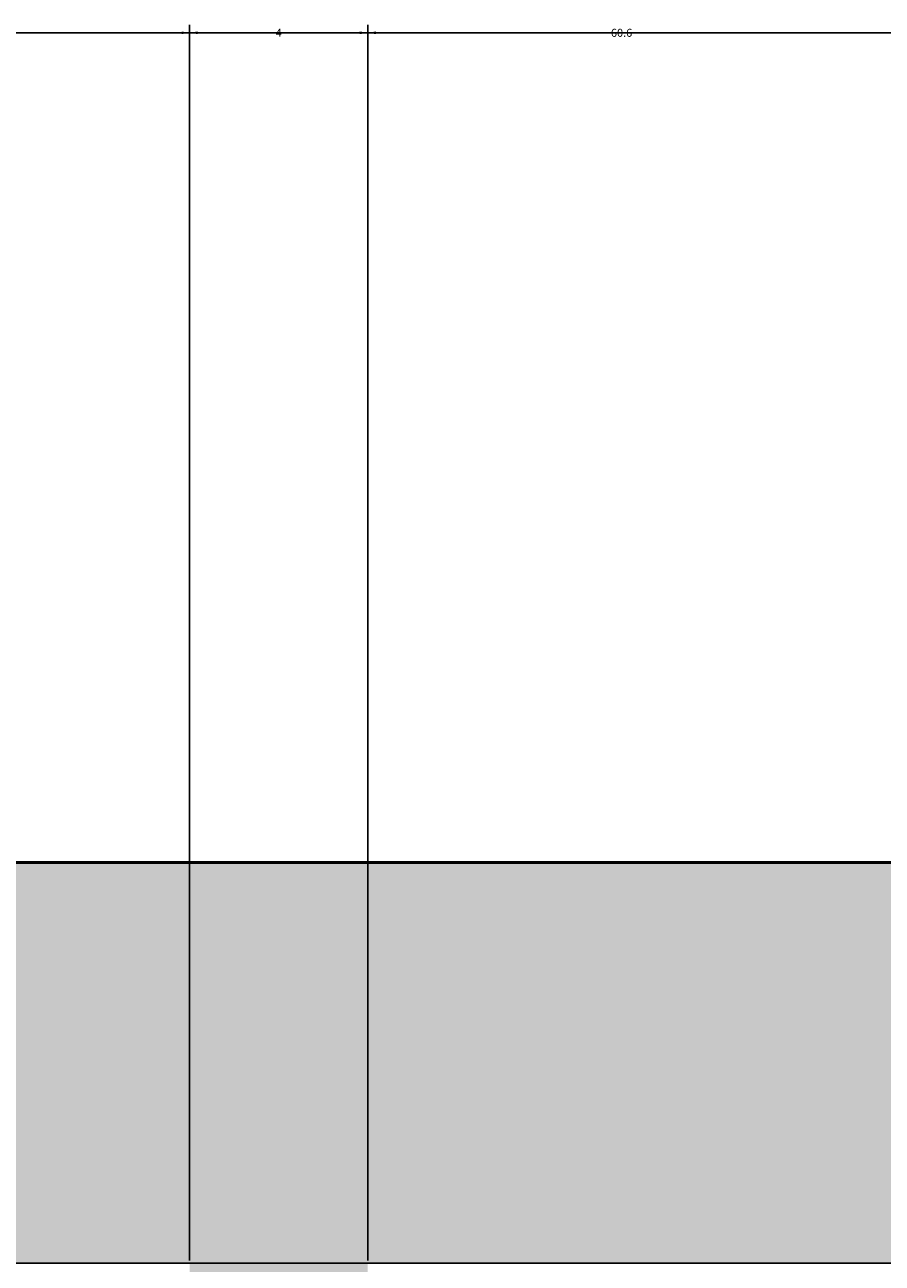
# Model space of a CAD drawing. Units: inches. Extents: x 2231 to 2461, y 2045 to 2455.
# Tile 88 of 95: x 2365 to 2384, y 2427 to 2455. Entities that reach past the tile are written whole.
import ezdxf

# ---------------------------------------------------------------- set-up
doc = ezdxf.new("R2010")
doc.units = ezdxf.units.IN
doc.layers.add('A-ANNO-DIMS', color=2, linetype='Continuous', lineweight=18)
doc.layers.add('A-WALL', color=7, linetype='Continuous', lineweight=50)
doc.layers.add('A-WALL-PATT', color=18, linetype='Continuous', lineweight=13, true_color=0x000000)
doc.styles.get("Standard").update_dxf_attribs({"font": 'arial.ttf'})
doc.dimstyles.get("Standard").update_dxf_attribs({"dimtxt": 0.18, "dimasz": 0.18, "dimexe": 0.18, "dimexo": 0.0625, "dimgap": 0.09, "dimtad": 0, "dimtih": 1, "dimtoh": 1, "dimdec": 4, "dimzin": 0, "dimdsep": 46, "dimtxsty": 'Standard', "dimcen": 0.09, "dimadec": 0, "dimazin": 0, "dimtfac": 1, "dimtdec": 4, "dimtofl": 0, "dimtmove": 0, "dimatfit": 3, "dimfxl": 1, "dimtolj": 1, "dimtzin": 0, "dimarcsym": 0})

# ---------------------------------------------------------------- blocks, each defined once
blk = doc.blocks.new('*D35')
at = {"layer": 'A-ANNO-DIMS', "color": 0, "lineweight": -2, "transparency": 16777216}
for p, q in [((2258.794, 2426.895), (2258.794, 2454.645)), ((2258.974, 2454.465), (2313.513, 2454.465)), ((2368.614, 2454.465), (2314.074, 2454.465)), ((2368.794, 2426.895), (2368.794, 2454.645))]:
    blk.add_line(p, q, dxfattribs=at)
at = {"layer": 'A-ANNO-DIMS', "color": 0, "transparency": 16777216}
for points in [[(2258.974, 2454.495), (2258.974, 2454.435), (2258.794, 2454.465)], [(2368.614, 2454.495), (2368.614, 2454.435), (2368.794, 2454.465)]]:
    blk.add_solid(points, dxfattribs=at)
at = {"layer": 'Defpoints', "color": 0, "transparency": 16777216}
for p in [(2368.794, 2454.465), (2258.794, 2426.833), (2368.794, 2426.833)]:
    blk.add_point(p, dxfattribs=at)
at = {"layer": 'A-ANNO-DIMS', "color": 0, "transparency": 16777216, "insert": (2313.794, 2454.465), "char_height": 0.18, "attachment_point": 5}
blk.add_mtext('\\A1;110', dxfattribs=at)
blk = doc.blocks.new('*D36')
at = {"layer": 'A-ANNO-DIMS', "color": 0, "lineweight": -2, "transparency": 16777216}
for p, q in [((2372.794, 2426.895), (2372.794, 2454.645)), ((2372.974, 2454.465), (2402.574, 2454.465)), ((2432.614, 2454.465), (2403.013, 2454.465)), ((2432.794, 2426.895), (2432.794, 2454.645))]:
    blk.add_line(p, q, dxfattribs=at)
at = {"layer": 'A-ANNO-DIMS', "color": 0, "transparency": 16777216}
for points in [[(2372.974, 2454.495), (2372.974, 2454.435), (2372.794, 2454.465)], [(2432.614, 2454.495), (2432.614, 2454.435), (2432.794, 2454.465)]]:
    blk.add_solid(points, dxfattribs=at)
at = {"layer": 'Defpoints', "color": 0, "transparency": 16777216}
for p in [(2432.794, 2454.465), (2372.794, 2426.833), (2432.794, 2426.833)]:
    blk.add_point(p, dxfattribs=at)
at = {"layer": 'A-ANNO-DIMS', "color": 0, "transparency": 16777216, "insert": (2402.794, 2454.465), "char_height": 0.18, "attachment_point": 5}
blk.add_mtext('\\A1;60', dxfattribs=at)
blk = doc.blocks.new('*D66')
at = {"layer": 'A-ANNO-DIMS', "color": 0, "lineweight": -2, "transparency": 16777216}
for p, q in [((2348.189, 2096.895), (2348.189, 2454.645)), ((2348.369, 2454.465), (2378.167, 2454.465)), ((2408.614, 2454.465), (2378.815, 2454.465)), ((2408.794, 2096.895), (2408.794, 2454.645))]:
    blk.add_line(p, q, dxfattribs=at)
at = {"layer": 'A-ANNO-DIMS', "color": 0, "transparency": 16777216}
for points in [[(2348.369, 2454.495), (2348.369, 2454.435), (2348.189, 2454.465)], [(2408.614, 2454.495), (2408.614, 2454.435), (2408.794, 2454.465)]]:
    blk.add_solid(points, dxfattribs=at)
at = {"layer": 'Defpoints', "color": 0, "transparency": 16777216}
for p in [(2408.794, 2454.465), (2348.189, 2096.833), (2408.794, 2096.833)]:
    blk.add_point(p, dxfattribs=at)
at = {"layer": 'A-ANNO-DIMS', "color": 0, "transparency": 16777216, "insert": (2378.491, 2454.465), "char_height": 0.18, "attachment_point": 5}
blk.add_mtext('\\A1;60.6', dxfattribs=at)
blk = doc.blocks.new('*D68')
at = {"layer": 'A-ANNO-DIMS', "color": 0, "lineweight": -2, "transparency": 16777216}
for p, q in [((2285.882, 2426.833), (2460.606, 2426.833)), ((2460.426, 2426.653), (2460.426, 2420.225)), ((2460.426, 2413.433), (2460.426, 2419.861)), ((2278.251, 2413.253), (2460.606, 2413.253))]:
    blk.add_line(p, q, dxfattribs=at)
at = {"layer": 'A-ANNO-DIMS', "color": 0, "transparency": 16777216}
for points in [[(2460.396, 2426.653), (2460.456, 2426.653), (2460.426, 2426.833)], [(2460.396, 2413.433), (2460.456, 2413.433), (2460.426, 2413.253)]]:
    blk.add_solid(points, dxfattribs=at)
at = {"layer": 'Defpoints', "color": 0, "transparency": 16777216}
for p in [(2285.82, 2426.833), (2460.426, 2426.833), (2278.188, 2413.253)]:
    blk.add_point(p, dxfattribs=at)
at = {"layer": 'A-ANNO-DIMS', "color": 0, "transparency": 16777216, "insert": (2460.426, 2420.043), "char_height": 0.18, "attachment_point": 5}
blk.add_mtext('\\A1;13.58', dxfattribs=at)
blk = doc.blocks.new('*D70')
at = {"layer": 'A-ANNO-DIMS', "color": 0, "lineweight": -2, "transparency": 16777216}
for p, q in [((2368.794, 2426.895), (2368.794, 2454.645)), ((2368.974, 2454.465), (2370.641, 2454.465)), ((2372.614, 2454.465), (2370.946, 2454.465)), ((2372.794, 2426.895), (2372.794, 2454.645))]:
    blk.add_line(p, q, dxfattribs=at)
at = {"layer": 'A-ANNO-DIMS', "color": 0, "transparency": 16777216}
for points in [[(2368.974, 2454.495), (2368.974, 2454.435), (2368.794, 2454.465)], [(2372.614, 2454.495), (2372.614, 2454.435), (2372.794, 2454.465)]]:
    blk.add_solid(points, dxfattribs=at)
at = {"layer": 'Defpoints', "color": 0, "transparency": 16777216}
for p in [(2372.794, 2454.465), (2368.794, 2426.833), (2372.794, 2426.833)]:
    blk.add_point(p, dxfattribs=at)
at = {"layer": 'A-ANNO-DIMS', "color": 0, "transparency": 16777216, "insert": (2370.794, 2454.465), "char_height": 0.18, "attachment_point": 5}
blk.add_mtext('\\A1;4', dxfattribs=at)

msp = doc.modelspace()

# ---------------------------------------------------------------- hatches: boundary and pattern name
at = {"layer": 'A-WALL-PATT'}
h = msp.add_hatch(color=256, dxfattribs=at)
h.dxf.hatch_style = 1
h.paths.add_polyline_path([(2441.7935, 2269.1535), (2432.7935, 2269.1535), (2432.7935, 2186.8328), (2396.7935, 2186.8328), (2396.7935, 2286.8328), (2394.7935, 2286.8328), (2394.7935, 2186.8328), (2334.7935, 2186.8328), (2334.7935, 2182.8328), (2432.7935, 2182.8328), (2432.7935, 2072.8328), (2416.6639, 2072.8328), (2416.6639, 2063.8328), (2441.7935, 2063.8328)])
h.paths.add_polyline_path([(2368.6639, 2072.8328), (2367.04, 2072.8328), (2330.7942, 2072.8328), (2330.7397, 2063.8328), (2368.6639, 2063.8328)])
h.paths.add_polyline_path([(2300.7392, 2068.3328), (2300.7392, 2072.8328), (2298.7935, 2072.8328), (2294.7935, 2072.8328), (2258.7935, 2072.8328), (2258.7935, 2120.8328), (2294.7935, 2120.8328), (2298.7935, 2120.8328), (2298.7935, 2128.8328), (2294.7935, 2128.8328), (2294.7935, 2124.8328), (2258.7935, 2124.8328), (2258.7935, 2182.8328), (2294.7935, 2182.8328), (2294.7935, 2174.8328), (2298.7935, 2174.8328), (2298.7935, 2182.8328), (2304.7935, 2182.8328), (2304.7935, 2186.8328), (2258.7935, 2186.8328), (2258.7935, 2221.999), (2249.7935, 2221.999), (2249.7935, 2063.8328), (2300.7392, 2063.8328)])
h.paths.add_polyline_path([(2391.9338, 2435.8328), (2333.82, 2435.8328), (2333.82, 2426.8328), (2368.7935, 2426.8328), (2368.7935, 2374.9508), (2368.7935, 2370.8328), (2372.3935, 2370.8328), (2372.7935, 2370.8328), (2372.7935, 2426.8328), (2391.9338, 2426.8328)])
h.paths.add_polyline_path([(2441.7935, 2435.8328), (2415.9338, 2435.8328), (2415.9338, 2426.8328), (2432.7935, 2426.8328), (2432.7935, 2334.8328), (2372.7935, 2334.8328), (2372.7935, 2346.8328), (2368.7935, 2346.8328), (2368.7935, 2306.8328), (2360.7935, 2306.8328), (2360.7935, 2302.8328), (2368.7935, 2302.8328), (2372.7935, 2302.8328), (2372.7935, 2330.8328), (2432.7935, 2330.8328), (2432.7935, 2317.1535), (2441.7935, 2317.1535)])
h.paths.add_polyline_path([(2285.82, 2435.8328), (2249.7935, 2435.8328), (2249.7935, 2269.999), (2258.7935, 2269.999), (2258.7935, 2302.8328), (2318.8168, 2302.8328), (2330.7935, 2302.8328), (2330.7935, 2306.8328), (2258.7935, 2306.8328), (2258.7935, 2426.8328), (2285.82, 2426.8328)])

# ---------------------------------------------------------------- linework, layer by layer
at = {"layer": 'A-WALL'}
msp.add_lwpolyline([(2300.7392, 2063.8328), (2249.7935, 2063.8328), (2249.7935, 2435.8328), (2441.7935, 2435.8328), (2441.7935, 2063.8328), (2330.7397, 2063.8328)], dxfattribs=at)

# ---------------------------------------------------------------- dimensions: what is measured, and where the dimension line sits
at = {"layer": 'A-ANNO-DIMS'}
for base, p1, p2, override, picture, middle in [((2368.7935, 2454.4653), (2258.7935, 2426.8328), (2368.7935, 2426.8328), {"dimdec": 0, "dimlfac": 1, "dimrnd": 0, "dimzin": 0, "dimdsep": 46, "dimlunit": 2}, '*D35', (2313.7935, 2454.4653)), ((2408.7935, 2454.4653), (2348.1888, 2096.8328), (2408.7935, 2096.8328), {"dimdec": 1, "dimlfac": 1, "dimrnd": 0, "dimzin": 0, "dimdsep": 46, "dimlunit": 2}, '*D66', (2378.4912, 2454.4653)), ((2372.7935, 2454.4653), (2368.7935, 2426.8328), (2372.7935, 2426.8328), {"dimdec": 0, "dimlfac": 1, "dimrnd": 0, "dimzin": 0, "dimdsep": 46, "dimlunit": 2}, '*D70', (2370.7935, 2454.4653)), ((2432.7935, 2454.4653), (2372.7935, 2426.8328), (2432.7935, 2426.8328), {"dimdec": 0, "dimlfac": 1, "dimrnd": 0, "dimzin": 0, "dimdsep": 46, "dimlunit": 2}, '*D36', (2402.7935, 2454.4653))]:
    dim = msp.add_linear_dim(base=base, p1=p1, p2=p2, dimstyle='Standard', override=override, dxfattribs=at)
    dim.commit()
    dim.dimension.update_dxf_attribs({"geometry": picture, "text_midpoint": middle})
dim = msp.add_linear_dim(base=(2460.426, 2426.8328), p1=(2278.1881, 2413.2534), p2=(2285.82, 2426.8328), angle=90, dimstyle='Standard', override={"dimdec": 2, "dimlfac": 1, "dimrnd": 0, "dimzin": 0, "dimdsep": 46, "dimlunit": 2}, dxfattribs=at)
dim.commit()
dim.dimension.update_dxf_attribs({"geometry": '*D68', "text_midpoint": (2460.426, 2420.0431)})

doc.saveas('drawing.dxf')
